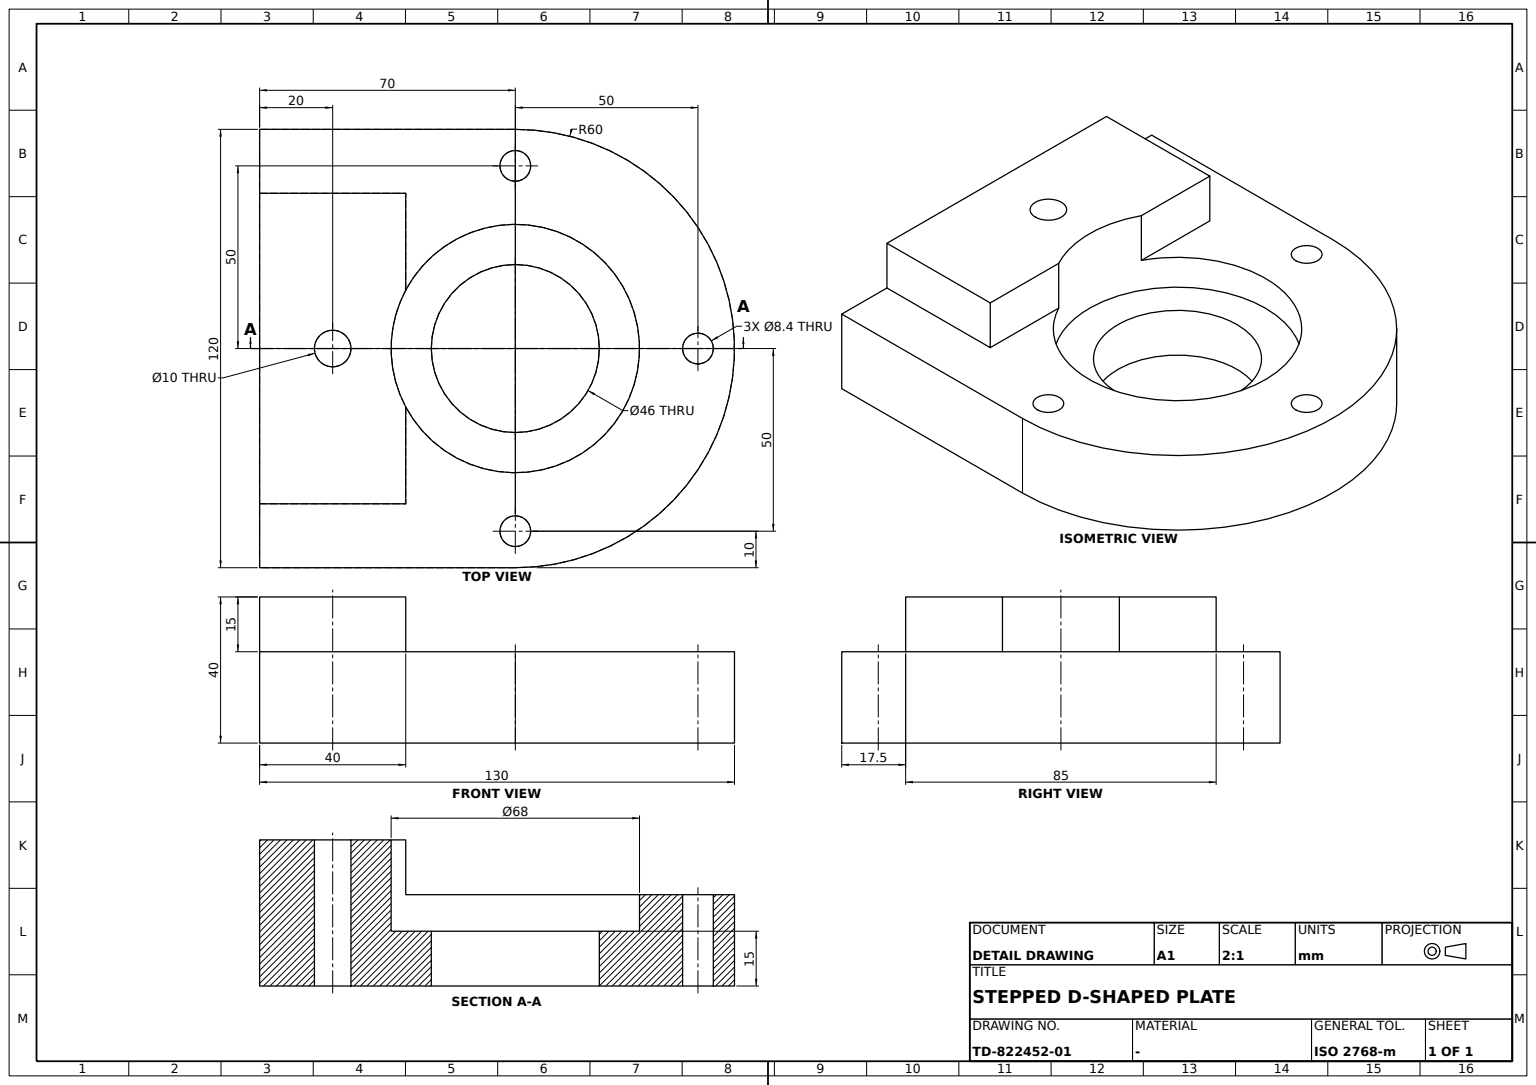
CATIA V5 part; units mm, degrees
sketch "Sketch1" plane through (0, 0, 0) normal (0, 0, 1) x (0, 1, 0)
  arc A0 (0, -60) -> (0, 60) centre (0, 0) ccw
  point P0 (0, 60)
  line L0 (0, 60) -> (-70, 60)
  point P1 (-70, 60)
  point P2 (-70, -60)
  point P3 (0, -60)
  line L1 (0, -60) -> (-70, -60)
  line L2 (-70, 60) -> (-70, -60)
  dimension "radius A0" = 60
  dimension "length L0" = 70
  constraint coincidence P0 y-axis
  constraint tangency L0 A0
  constraint symmetry P1 P2 x-axis
  constraint symmetry P0 P3 x-axis
  constraint symmetry L0 L1 x-axis
  constraint vertical L2 y-axis
extrude "Pad1" add sketch "Sketch1" along normal blind 25
sketch "Sketch2" plane through (0, 0, 25) normal (0, 0, 1) x (0, 1, 0)
  line L0 (-70, 42.5) -> (-30, 42.5)
  line L1 (-30, 42.5) -> (-30, -42.5)
  line L2 (-30, -42.5) -> (-70, -42.5)
  line L3 (-70, -42.5) -> (-70, 42.5)
  line L4 (-70, 60) -> (-70, -60) construction
  dimension "length L0" = 40
  dimension "length L1" = 85
  dimension "D3" = 42.5
  constraint horizontal L0 x-axis
  constraint horizontal L2 x-axis
  constraint vertical L1 y-axis
  constraint vertical L3 y-axis
  constraint coincidence L3 L4
extrude "Pad2" add sketch "Sketch2" along normal blind 15
sketch "Sketch3" plane through (-13.5166, 37.4414, 25) normal (0, 0, 1) x (1, 0, 0)
  point P0 (13.5166, -37.4414)
  arc A0 (73.5166, -37.4414) -> (-46.4834, -37.4414) centre (13.5166, -37.4414) ccw construction
  constraint concentricity A0 P0
hole "Hole1" at (0, 0, 25) direction (0, 0, -1) diameter 68 depth 10
sketch "Sketch4" plane through (0, 0, 15) normal (0, 0, 1) x (1, 0, 0)
  point P0 (0, 0)
hole "Hole2" at (0, 0, 15) direction (0, 0, -1) diameter 46 depth 25
sketch "Sketch5" plane through (0, 0, 40) normal (0, 0, 1) x (0, 1, 0)
  circle A0 centre (-50, 0) radius 5
  point P0 (-50, 0)
  line L0 (-70, 42.5) -> (-70, -42.5) construction
  dimension "radius A0" = 5
  dimension "distance P0 L0" = 20
  constraint coincidence P0 x-axis
extrude "Pocket1" cut sketch "Sketch5" against normal up to next
sketch "Sketch6" plane through (0, 0, 25) normal (0, 0, 1) x (0, 1, 0)
  arc A0 (0, -50) -> (0, 50) centre (0, 0) ccw construction
  point P0 (0, 73.3712)
  circle A1 centre (0, 50) radius 4.2023
  circle A2 centre (50, 0) radius 4.2023
  point P1 (50, 0)
  circle A3 centre (0, -50) radius 4.2023
  dimension "radius A0" = 50
  dimension "radius A1" = 4.2023
  dimension "radius A2" = 4.2023
  dimension "radius A3" = 4.2023
  constraint coincidence P0 y-axis
  constraint coincidence P1 A0
  constraint coincidence P1 x-axis
extrude "Pocket2" cut sketch "Sketch6" against normal up to next
properties part number "catia 18"
